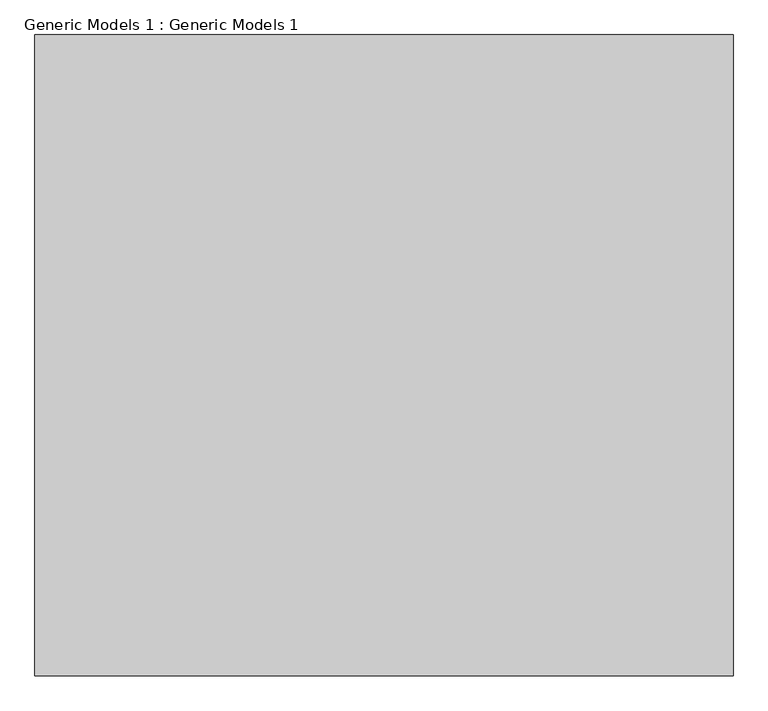
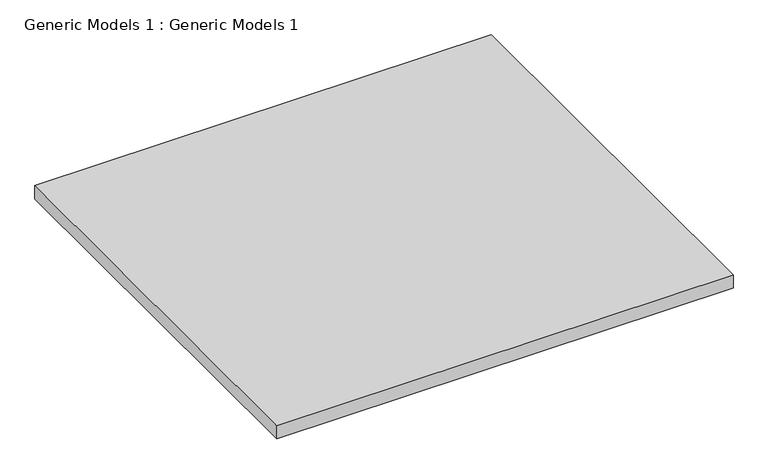
"""IFC4 building model written with IfcOpenShell, lengths in millimetres: proxy geometry, Generic Models 1 : Generic Models 1."""

from ifc_helpers import new_model, si_unit, frame, origin, place, context, project, spatial, polyline, outline, extrude, source, transform, mapped, element, save


def generic_models_1_generic_models_1_ab7b9371(model_context):
    return source(origin(), model_context, "Body", "SweptSolid", [
        extrude(outline(polyline([(1235.2423568, -5561.671685), (11295.1692178, -5561.671685), (11295.1692178, -14801.9914627), (1235.2423568, -14801.9914627), (1235.2423568, -5561.671685)])), frame((0.0, 0.0, 9448.8), z_axis=(0.0, 0.0, 1.0), x_axis=(1.0, 0.0, 0.0)), (0.0, 0.0, 1.0), 304.8),
    ])


if __name__ == "__main__":
    model = new_model("IFC4")
    model_context = context("Model", 3, world=origin())
    ifc_project = project(units=[si_unit("LENGTHUNIT", "METRE", prefix="MILLI")], contexts=[model_context])
    site = spatial("IfcSite", under=ifc_project)
    building = spatial("IfcBuilding", under=site)
    placement = place(None, origin())
    generic_models_1_generic_models_1_shape = generic_models_1_generic_models_1_ab7b9371(model_context)
    element("IfcBuildingElementProxy", 1, Name="Generic Models 1 : Generic Models 1", ObjectType="Generic Models 1 : Generic Models 1", at=placement, inside=building, context=model_context, shape_type="MappedRepresentation", body=[
        mapped(generic_models_1_generic_models_1_shape, transform((0.0, 0.0, 0.0), x_axis=(1.0, 0.0, 0.0), y_axis=(0.0, 1.0, 0.0), z_axis=(0.0, 0.0, 1.0))),
    ])
    save(model, "model.ifc")

# Revit data of these elements
# Element 1 (IfcBuildingElementProxy, "Generic Models 1 : Generic Models 1")
#   Materials on its faces: "Clad - White"
# Materials
#   "Clad - White": class "Wood", colour RGB 242 242 238, transparency 0, Cost = 0
